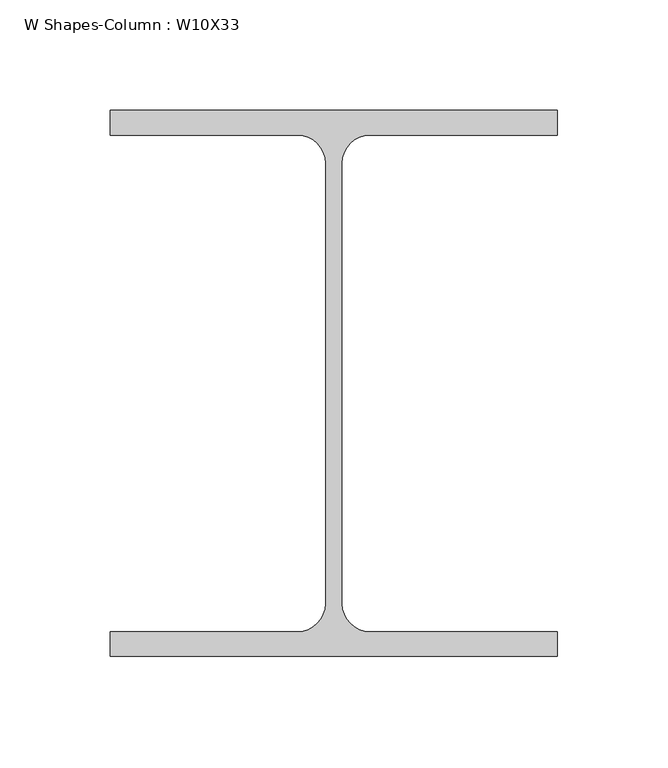
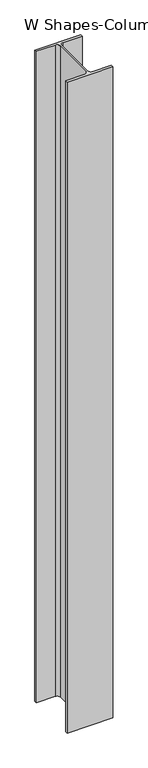
"""IFC4 building model written with IfcOpenShell, lengths in millimetres: column geometry, W Shapes-Column : W10X33."""

from ifc_helpers import new_model, si_unit, point, frame, frame_2d, origin, place, context, project, spatial, polyline, circle_curve, trimmed, segment, composite_curve, outline, extrude, source, transform, mapped, element, save


def w_shapes_column_w10x33_9bdcd76c(model_context):
    return source(origin(), model_context, "Body", "SweptSolid", [
        extrude(outline(composite_curve([segment(polyline([(101.092, 123.571), (101.092, 112.395), (16.383, 112.395)]), True, "CONTINUOUS"), segment(trimmed(circle_curve(frame_2d((16.383, 99.695)), 12.7), [point((16.383, 112.395))], [point((3.683, 99.695))], True, "CARTESIAN"), True, "CONTINUOUS"), segment(polyline([(3.683, 99.695), (3.683, -99.695)]), True, "CONTINUOUS"), segment(trimmed(circle_curve(frame_2d((16.383, -99.695)), 12.7), [point((3.683, -99.695))], [point((16.383, -112.395))], True, "CARTESIAN"), True, "CONTINUOUS"), segment(polyline([(16.383, -112.395), (101.092, -112.395), (101.092, -123.571), (-101.092, -123.571), (-101.092, -112.395), (-16.383, -112.395)]), True, "CONTINUOUS"), segment(trimmed(circle_curve(frame_2d((-16.383, -99.695)), 12.7), [point((-16.383, -112.395))], [point((-3.683, -99.695))], True, "CARTESIAN"), True, "CONTINUOUS"), segment(polyline([(-3.683, -99.695), (-3.683, 99.695)]), True, "CONTINUOUS"), segment(trimmed(circle_curve(frame_2d((-16.383, 99.695)), 12.7), [point((-3.683, 99.695))], [point((-16.383, 112.395))], True, "CARTESIAN"), True, "CONTINUOUS"), segment(polyline([(-16.383, 112.395), (-101.092, 112.395), (-101.092, 123.571), (101.092, 123.571)]), True, "CONTINUOUS")], self_intersect=False)), frame((0.0, 0.0, 3048.0), z_axis=(0.0, 0.0, 1.0), x_axis=(1.0, 0.0, 0.0)), (0.0, 0.0, 1.0), 3048.0),
    ])


if __name__ == "__main__":
    model = new_model("IFC4")
    model_context = context("Model", 3, world=origin())
    ifc_project = project(units=[si_unit("LENGTHUNIT", "METRE", prefix="MILLI")], contexts=[model_context])
    site = spatial("IfcSite", under=ifc_project)
    building = spatial("IfcBuilding", under=site)
    placement = place(None, origin())
    w_shapes_column_w10x33_shape = w_shapes_column_w10x33_9bdcd76c(model_context)
    element("IfcColumn", 1, ObjectType="W Shapes-Column : W10X33", at=placement, inside=building, context=model_context, shape_type="MappedRepresentation", body=[
        mapped(w_shapes_column_w10x33_shape, transform((0.0, 0.0, 0.0), x_axis=(1.0, 0.0, 0.0), y_axis=(0.0, 1.0, 0.0), z_axis=(0.0, 0.0, 1.0))),
    ])
    save(model, "model.ifc")

# Revit data of these elements
# Type "W Shapes-Column : W10X33"
#   Section Name Key = "W10x33"
#   Assembly Code = "B10"
#   Width = 7.960"
#   Web Thickness = 0.290"
#   Web Fillet = 0.500"
#   Warping Constant = 791.00 in⁶
#   Torsional Moment of Inertia = 0.583 in⁴
#   Section Area = 9.71 in²
#   Plastic Modulus weak axis = 14.00 in³
#   Plastic Modulus strong axis = 38.80 in³
#   Perimeter = 49.90 ft²/ft
#   Nominal Weight = 33.00 lbf/ft
#   Moment of Inertia weak axis = 36.60 in⁴
#   Moment of Inertia strong axis = 171.00 in⁴
#   Height = 9.730"
#   Flange Thickness = 0.440"
#   Elastic Modulus weak axis = 9.20 in³
#   Elastic Modulus strong axis = 35.00 in³
#   Centroid Vertical = 4.865"
#   Centroid Horizontal = 3.980"
#   Structural Material [instance default] = Steel ASTM A992
#   Principal Axes Angle = 0
# Element 1 (IfcColumn, "W Shapes-Column : W10X33")
#   Materials on its faces: "Steel ASTM A992"
# Materials
#   "Steel ASTM A992": class "Metal", colour RGB 199 199 199, transparency 0, Description = "Structural steel 50ksi", Cost = 0
